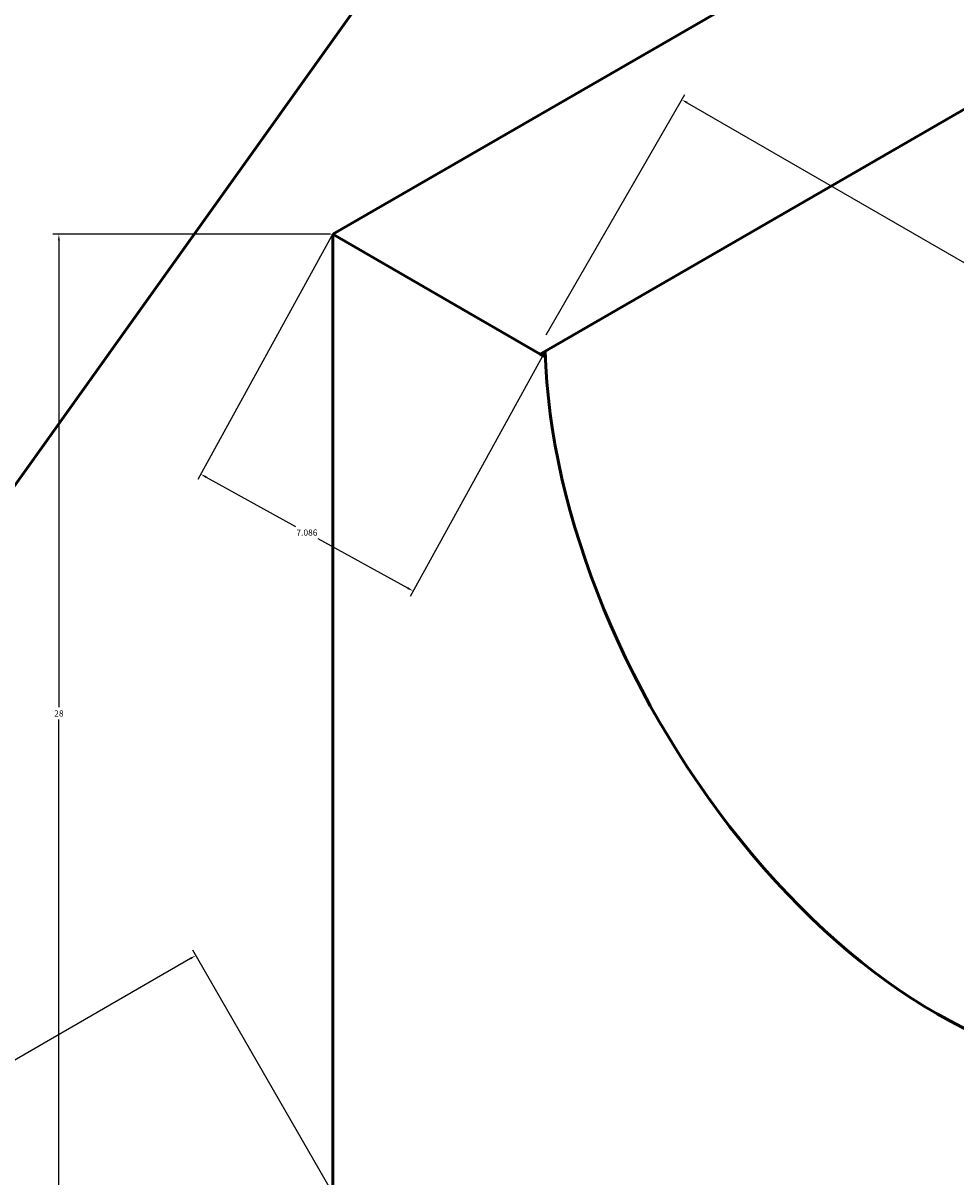
# Model space of a CAD drawing. Units: millimetres. Extents: x 2919 to 3075, y 2801 to 2951.
# Tile 5 of 14: x 2952 to 2979, y 2876 to 2910. Entities that reach past the tile are written whole.
import ezdxf

# ---------------------------------------------------------------- set-up
doc = ezdxf.new("R2010")
doc.units = ezdxf.units.MM
doc.layers.add('M-DIMS', color=2, linetype='Continuous', lineweight=18)
doc.layers.add('M-OUTL', color=7, linetype='Continuous', lineweight=50)
doc.styles.get("Standard").update_dxf_attribs({"font": 'arial.ttf'})
doc.dimstyles.get("Standard").update_dxf_attribs({"dimtxt": 0.18, "dimasz": 0.18, "dimexe": 0.18, "dimexo": 0.0625, "dimgap": 0.09, "dimtad": 0, "dimtih": 1, "dimtoh": 1, "dimdec": 4, "dimzin": 0, "dimdsep": 46, "dimtxsty": 'Standard', "dimcen": 0.09, "dimadec": 0, "dimazin": 0, "dimtfac": 1, "dimtdec": 4, "dimtofl": 0, "dimtmove": 0, "dimatfit": 3, "dimfxl": 1, "dimtolj": 1, "dimtzin": 0, "dimarcsym": 0})

# ---------------------------------------------------------------- blocks, each defined once
blk = doc.blocks.new('*D10')
at = {"layer": 'Defpoints', "color": 0, "transparency": 16777216}
for p in [(2956.682, 2882.821), (2960.682, 2875.893), (2941.63, 2864.893)]:
    blk.add_point(p, dxfattribs=at)
at = {"layer": 'M-DIMS', "color": 0, "lineweight": -2, "transparency": 16777216}
for p, q in [((2956.526, 2882.731), (2947.375, 2877.448)), ((2960.651, 2875.947), (2956.592, 2882.977)), ((2937.785, 2871.911), (2946.936, 2877.195)), ((2941.598, 2864.947), (2937.54, 2871.977))]:
    blk.add_line(p, q, dxfattribs=at)
at = {"layer": 'M-DIMS', "color": 0, "transparency": 16777216}
for points in [[(2956.511, 2882.757), (2956.541, 2882.705), (2956.682, 2882.821)], [(2937.77, 2871.937), (2937.8, 2871.885), (2937.63, 2871.821)]]:
    blk.add_solid(points, dxfattribs=at)
at = {"layer": 'M-DIMS', "color": 0, "transparency": 16777216, "insert": (2947.156, 2877.321), "char_height": 0.18, "attachment_point": 5}
blk.add_mtext('\\A1;22', dxfattribs=at)
blk = doc.blocks.new('*D13')
at = {"layer": 'Defpoints', "color": 0, "transparency": 16777216}
for p in [(2952.682, 2903.893), (2960.682, 2903.893), (2960.682, 2875.893)]:
    blk.add_point(p, dxfattribs=at)
at = {"layer": 'M-DIMS', "color": 0, "lineweight": -2, "transparency": 16777216}
for p, q in [((2960.62, 2903.893), (2952.502, 2903.893)), ((2952.682, 2903.713), (2952.682, 2890.075)), ((2952.682, 2876.073), (2952.682, 2889.711)), ((2960.62, 2875.893), (2952.502, 2875.893))]:
    blk.add_line(p, q, dxfattribs=at)
at = {"layer": 'M-DIMS', "color": 0, "transparency": 16777216}
for points in [[(2952.652, 2903.713), (2952.712, 2903.713), (2952.682, 2903.893)], [(2952.652, 2876.073), (2952.712, 2876.073), (2952.682, 2875.893)]]:
    blk.add_solid(points, dxfattribs=at)
at = {"layer": 'M-DIMS', "color": 0, "transparency": 16777216, "insert": (2952.682, 2889.893), "char_height": 0.18, "attachment_point": 5}
blk.add_mtext('\\A1;28', dxfattribs=at)
blk = doc.blocks.new('*D17')
at = {"layer": 'Defpoints', "color": 0, "transparency": 16777216}
for p in [(2966.884, 2900.897), (2993.691, 2894.658), (2989.691, 2887.729)]:
    blk.add_point(p, dxfattribs=at)
at = {"layer": 'M-DIMS', "color": 0, "lineweight": -2, "transparency": 16777216}
for p, q in [((2966.915, 2900.951), (2970.974, 2907.981)), ((2971.04, 2907.735), (2981.964, 2901.428)), ((2993.535, 2894.748), (2982.611, 2901.054)), ((2989.722, 2887.783), (2993.781, 2894.813))]:
    blk.add_line(p, q, dxfattribs=at)
at = {"layer": 'M-DIMS', "color": 0, "transparency": 16777216}
for points in [[(2971.055, 2907.761), (2971.025, 2907.709), (2970.884, 2907.825)], [(2993.55, 2894.774), (2993.52, 2894.722), (2993.691, 2894.658)]]:
    blk.add_solid(points, dxfattribs=at)
at = {"layer": 'M-DIMS', "color": 0, "transparency": 16777216, "insert": (2982.287, 2901.241), "char_height": 0.18, "attachment_point": 5}
blk.add_mtext('\\A1;%%c26.334', dxfattribs=at)
blk = doc.blocks.new('*D20')
at = {"layer": 'Defpoints', "color": 0, "transparency": 16777216}
for p in [(2960.682, 2903.893), (2966.89, 2900.477), (2956.825, 2896.884)]:
    blk.add_point(p, dxfattribs=at)
at = {"layer": 'M-DIMS', "color": 0, "lineweight": -2, "transparency": 16777216}
for p, q in [((2960.652, 2903.838), (2956.739, 2896.727)), ((2966.86, 2900.423), (2962.946, 2893.311)), ((2956.983, 2896.798), (2959.599, 2895.358)), ((2962.875, 2893.555), (2960.26, 2894.994))]:
    blk.add_line(p, q, dxfattribs=at)
at = {"layer": 'M-DIMS', "color": 0, "transparency": 16777216}
for points in [[(2956.998, 2896.824), (2956.969, 2896.771), (2956.825, 2896.884)], [(2962.89, 2893.581), (2962.861, 2893.529), (2963.033, 2893.468)]]:
    blk.add_solid(points, dxfattribs=at)
at = {"layer": 'M-DIMS', "color": 0, "transparency": 16777216, "insert": (2959.929, 2895.176), "char_height": 0.18, "attachment_point": 5}
blk.add_mtext('\\A1;7.086', dxfattribs=at)

msp = doc.modelspace()

# ---------------------------------------------------------------- linework, layer by layer
at = {"layer": 'M-OUTL'}
for p, q in [((2960.6821, 2903.8932), (2995.3232, 2923.8932)), ((2966.7443, 2900.3932), (3001.3853, 2920.3932)), ((2960.6821, 2875.8932), (2960.6821, 2903.8932)), ((2960.6821, 2903.8932), (2966.7443, 2900.3932)), ((2966.7443, 2900.3932), (2966.8952, 2900.3138))]:
    msp.add_line(p, q, dxfattribs=at)
msp.add_lwpolyline([(2941.6296, 2882.8932), (2961.6296, 2910.8932), (2995.3232, 2930.3462)], dxfattribs=at)
msp.add_lwpolyline([(2941.6296, 2882.8932), (2961.6296, 2910.8932), (2995.3232, 2930.3462)], dxfattribs=at)
msp.add_ellipse((2978.2874, 2894.3129), major_axis=(8.0632, -13.966), ratio=0.5773503, start_param=3.9585863, end_param=7.1123769, dxfattribs=at)

# ---------------------------------------------------------------- dimensions: what is measured, and where the dimension line sits
at = {"layer": 'M-DIMS'}
dim = msp.add_linear_dim(base=(2993.69055, 2894.65752), p1=(2966.88424, 2900.89655), p2=(2989.69055, 2887.72932), angle=330, text='%%c<>', dimstyle='Standard', override={"dimdec": 3, "dimlfac": 1, "dimrnd": 0, "dimzin": 0, "dimdsep": 46, "dimlunit": 2}, dxfattribs=at)
dim.commit()
dim.dimension.update_dxf_attribs({"geometry": '*D17', "text_midpoint": (2982.2874, 2901.24114)})
for base, p1, p2, angle, override, picture, middle in [((2952.6821, 2903.8932), (2960.6821, 2875.8932), (2960.6821, 2903.8932), 90, {"dimdec": 0, "dimlfac": 1, "dimrnd": 0, "dimzin": 0, "dimdsep": 46, "dimlunit": 2}, '*D13', (2952.6821, 2889.8932)), ((2956.8254, 2896.8843), (2966.8899, 2900.4773), (2960.6821, 2903.8932), 151.17749, {"dimdec": 3, "dimlfac": 1, "dimrnd": 0, "dimzin": 0, "dimdsep": 46, "dimlunit": 2}, '*D20', (2959.9293, 2895.1763)), ((2956.6821, 2882.8214), (2941.6296, 2864.8932), (2960.6821, 2875.8932), 30, {"dimdec": 0, "dimlfac": 1, "dimrnd": 0, "dimzin": 0, "dimdsep": 46, "dimlunit": 2}, '*D10', (2947.1559, 2877.3214))]:
    dim = msp.add_linear_dim(base=base, p1=p1, p2=p2, angle=angle, dimstyle='Standard', override=override, dxfattribs=at)
    dim.commit()
    dim.dimension.update_dxf_attribs({"geometry": picture, "text_midpoint": middle})

doc.saveas('drawing.dxf')
